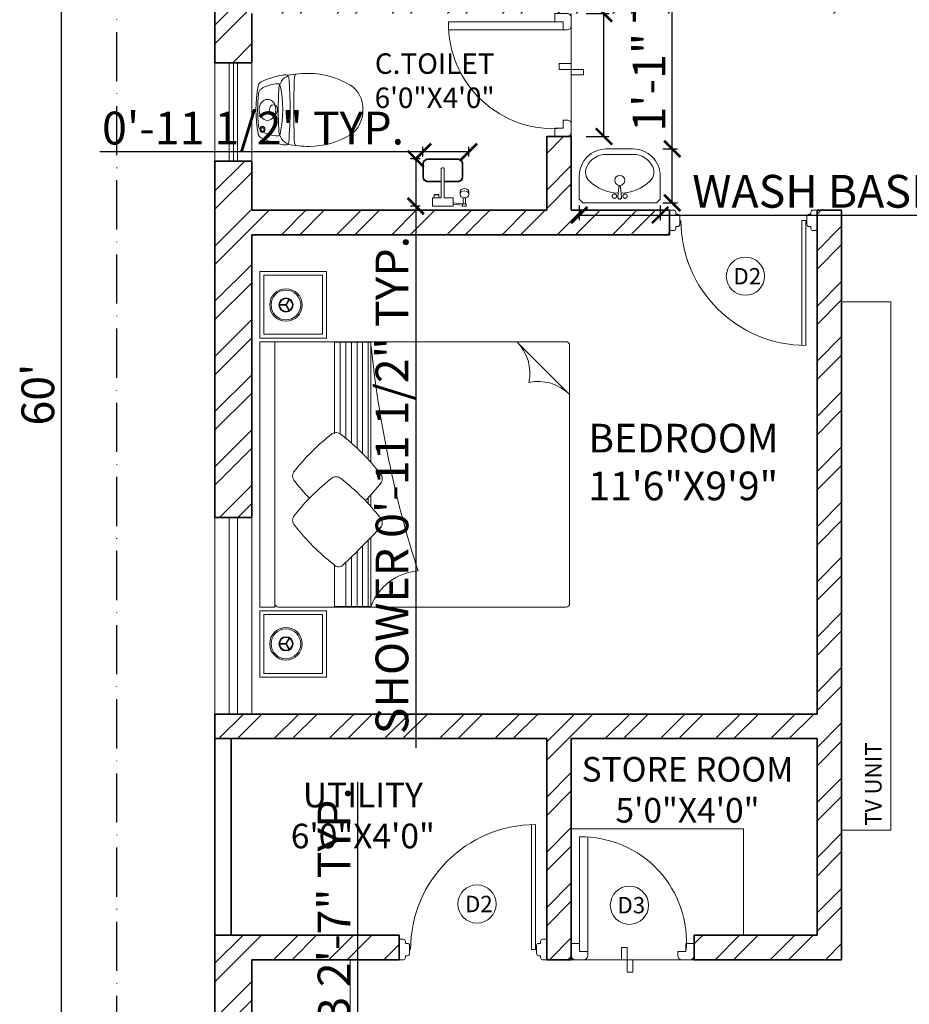
# Model space of a CAD drawing. Units: inches. Extents: x -15 to 1053, y -1 to 793.
# Tile 5 of 8: x 595 to 813, y 256 to 496. Entities that reach past the tile are written whole.
import ezdxf

# ---------------------------------------------------------------- set-up
doc = ezdxf.new("R2010")
doc.units = ezdxf.units.IN
doc.linetypes.add('ACAD_ISO10W100', pattern=[18, 12, -3, 0, -3])
for name, color, linetype, lineweight in [('00 FURNITURE', 15, 'Continuous', 15), ('A-ANNO-DIMS', 2, 'Continuous', 18), ('A-ANNO-TEXT', 7, 'Continuous', 18), ('A-AREA-IDEN', 7, 'Continuous', 18), ('A-DOOR', 4, 'Continuous', 18), ('A-FLOR-CASE', 5, 'Continuous', 18), ('A-FLOR-FIXT', 8, 'Continuous', 13), ('A-FURN', 8, 'Continuous', 13), ('A-GLAZ', 4, 'Continuous', 18), ('A-WALL', 7, 'Continuous', 35), ('A-WALL-PATT', 8, 'Continuous', 13), ('A_FUR 1', 5, 'Continuous', 5), ('C-PROP', 1, 'ACAD_ISO10W100', 25)]:
    doc.layers.add(name, color=color, linetype=linetype, lineweight=lineweight)
doc.styles.add('1-100DIM', font='txt', dxfattribs={"height": 0.3})
doc.styles.get("Standard").update_dxf_attribs({"font": 'arial.ttf'})
doc.dimstyles.new('ISO-25', dxfattribs={"dimtxt": 8, "dimasz": 4, "dimexe": 1.25, "dimexo": 0.625, "dimtad": 1, "dimdec": 0, "dimlunit": 4, "dimtxsty": 'Standard', "dimblk": 'ARCHTICK', "dimcen": 3, "dimadec": 0, "dimazin": 0, "dimtfac": 1, "dimtdec": 0, "dimtmove": 0, "dimatfit": 3, "dimldrblk": 'ARCHTICK', "dimfxl": 1, "dimarcsym": 0})

# ---------------------------------------------------------------- blocks, each defined once
blk = doc.blocks.new('_ArchTick')
at = {"color": 0, "linetype": 'ByBlock', "const_width": 0.15}
blk.add_lwpolyline([(-0.5, -0.5), (0.5, 0.5)], dxfattribs=at)
blk = doc.blocks.new('*D19')
at = {"layer": 'A-ANNO-DIMS', "color": 0, "lineweight": -2, "transparency": 16777216}
for p, q in [((618.45, 764.76), (604.32, 764.76)), ((605.57, 764.76), (605.57, 44.76)), ((618.45, 44.76), (604.32, 44.76))]:
    blk.add_line(p, q, dxfattribs=at)
at = {"layer": 'Defpoints', "color": 0, "transparency": 16777216}
for p in [(619.07, 764.76), (605.57, 44.76), (619.07, 44.76)]:
    blk.add_point(p, dxfattribs=at)
at = {"layer": 'A-ANNO-DIMS', "color": 0, "lineweight": -2, "transparency": 16777216, "xscale": 4, "yscale": 4, "zscale": 4}
for p, rotation in [((605.57, 764.76), 90), ((605.57, 44.76), 270)]:
    blk.add_blockref('_ArchTick', p, dxfattribs=dict(at, rotation=rotation))
at = {"layer": 'A-ANNO-DIMS', "color": 0, "transparency": 16777216, "insert": (600.86, 404.76), "char_height": 8, "attachment_point": 5, "rotation": 90}
blk.add_mtext("60'", dxfattribs=at)
blk = doc.blocks.new('ESTSET')
at = {"layer": 'A_FUR 1'}
for p, q in [((-10.44, 4.1), (-10.44, 32.1)), ((-8.44, 4.1), (-8.44, 32.1)), ((-36.44, 6.1), (-36.44, 3.1)), ((-34.44, 6.1), (-36.44, 6.1)), ((-34.44, 4.1), (-34.44, 6.1)), ((-34.44, 4.1), (-34.44, 6.1)), ((-8.44, 4.1), (-8.44, 6.1)), ((-8.44, 6.1), (-6.44, 6.1)), ((-8.44, 4.1), (-8.44, 6.1)), ((-6.44, 6.1), (-6.44, 3.1)), ((-32.44, 4.1), (-34.44, 4.1)), ((-32.44, 4.1), (-34.44, 4.1)), ((-32.44, 3.1), (-32.44, 4.1)), ((-10.44, 3.1), (-10.44, 4.1)), ((-10.44, 4.1), (-8.44, 4.1)), ((-10.44, 4.1), (-8.44, 4.1)), ((-6.44, 2.1), (-36.44, 2.1)), ((-35.44, 2.1), (-33.44, 2.1)), ((-7.44, 2.1), (-9.44, 2.1))]:
    blk.add_line(p, q, dxfattribs=at)
for points in [[(-21.44, 2.1), (-18.67, 2.1), (-18.67, 5.1), (-20.06, 5.1)], [(-20.06, 5.1), (-20.06, -0.91)], [(-21.44, 2.1), (-21.44, -0.91), (-20.06, -0.91)]]:
    blk.add_lwpolyline(points, dxfattribs=at)
for centre, radius, start, end in [((-8.91, 6.46), 25.64, 88.9606, 185.2816), ((-35.44, 3.1), 1, 180, 270), ((-33.44, 3.1), 1, 270, 0), ((-9.44, 3.1), 1, 180, 270), ((-7.44, 3.1), 1, 270, 0)]:
    blk.add_arc(centre, radius, start, end, dxfattribs=at)
blk = doc.blocks.new('RGWTG')
at = {"layer": '00 FURNITURE'}
for p, q in [((578.23, 3473.51), (577.36, 3475.01)), ((578.23, 3473.58), (577.36, 3472.08)), ((578.36, 3473.58), (577.49, 3475.09)), ((578.29, 3473.62), (580.03, 3473.62)), ((578.36, 3473.51), (577.49, 3472)), ((578.29, 3473.47), (580.03, 3473.47)), ((521.93, 3464.58), (509.03, 3451.68)), ((509.93, 3464.58), (566.4, 3464.58)), ((557.53, 3463.84), (557.53, 3464.49)), ((557.53, 3464.49), (566.4, 3464.49)), ((558.2, 3464.49), (558.2, 3435.82)), ((559.57, 3464.49), (559.57, 3437.25)), ((560.94, 3464.49), (560.94, 3438.58)), ((562.3, 3464.49), (562.3, 3439.83)), ((563.67, 3464.49), (563.67, 3440.99)), ((565.04, 3464.49), (565.04, 3442.08)), ((566.4, 3464.58), (580.98, 3464.58)), ((566.4, 3464.49), (566.4, 3442.08)), ((566.4, 3464.49), (566.4, 3463.84)), ((580.98, 3464.58), (580.98, 3416.72)), ((509.03, 3422.63), (509.03, 3463.68)), ((558.2, 3426.48), (558.2, 3425.04)), ((509.03, 3400.68), (509.03, 3422.63)), ((558.2, 3416.13), (558.2, 3399.95)), ((580.98, 3416.72), (580.98, 3400.68)), ((559.57, 3414.75), (559.57, 3399.95)), ((560.94, 3413.39), (560.94, 3399.95)), ((562.3, 3412.04), (562.3, 3399.95)), ((563.67, 3410.72), (563.67, 3399.95)), ((580.08, 3399.78), (509.93, 3399.78)), ((557.53, 3399.95), (557.53, 3400.6)), ((566.4, 3399.95), (557.53, 3399.95)), ((566.4, 3400.6), (566.4, 3399.95)), ((578.23, 3390.78), (577.36, 3392.29)), ((578.36, 3390.86), (577.49, 3392.36)), ((578.23, 3390.86), (577.36, 3389.36)), ((578.36, 3390.78), (577.49, 3389.28)), ((578.29, 3390.9), (580.03, 3390.9)), ((578.29, 3390.74), (580.03, 3390.74))]:
    blk.add_line(p, q, dxfattribs=at)
for points in [[(568.43, 3465.48), (584.63, 3465.48), (584.63, 3481.68), (568.43, 3481.68)], [(569.33, 3466.38), (583.73, 3466.38), (583.73, 3480.78), (569.33, 3480.78)], [(580.98, 3399.78), (584.63, 3399.78), (584.63, 3464.58), (580.98, 3464.58)], [(568.43, 3398.88), (584.63, 3398.88), (584.63, 3382.68), (568.43, 3382.68)], [(569.33, 3397.98), (583.73, 3397.98), (583.73, 3383.58), (569.33, 3383.58)]]:
    blk.add_lwpolyline(points, close=True, dxfattribs=at)
for points in [[(566.52, 3464.49), (557.53, 3464.49), (557.53, 3435.08)], [(557.53, 3427.21), (557.53, 3424.3)], [(557.53, 3416.82), (557.53, 3399.95), (566.4, 3399.95), (566.4, 3409.94)]]:
    blk.add_lwpolyline(points, dxfattribs=at)
for centre, radius in [((578.29, 3473.54), 3.97), ((578.29, 3473.54), 3.63), ((578.29, 3473.54), 1.74), ((578.29, 3473.54), 1.56), ((578.29, 3390.82), 3.97), ((578.29, 3390.82), 3.63), ((578.29, 3390.82), 1.74), ((578.29, 3390.82), 1.56)]:
    blk.add_circle(centre, radius, dxfattribs=at)
for centre, radius, start, end in [((509.93, 3463.68), 0.9, 90, 180), ((529.65, 3456.88), 10.9, 135.0361, 191.9278), ((290.56, 3490.52), 268.3, 342.2214, 354.2925), ((516.73, 3443.97), 10.9, 78.0722, 134.9639), ((566.05, 3440.57), 1.82, 45, 135), ((598.15, 3399.01), 54.32, 127.931, 142.069), ((533.58, 3399.31), 54.32, 37.931, 52.069), ((574.84, 3431.77), 1.82, 315, 45), ((556.59, 3431.11), 1.82, 135, 225), ((598.15, 3388.23), 54.32, 127.931, 142.069), ((566.05, 3429.78), 1.82, 45, 135), ((533.58, 3388.53), 54.32, 37.931, 52.069), ((533.28, 3463.88), 54.32, 316.32, 322.069), ((597.87, 3463.6), 54.32, 217.931, 224.141), ((556.59, 3420.33), 1.82, 135, 225), ((574.84, 3420.99), 1.82, 315, 45), ((765.33, 3619.75), 290.45, 223.6069, 226.2326), ((533.28, 3453.1), 54.32, 307.931, 322.069), ((565.44, 3411.05), 1.47, 225.9674, 326.8337), ((545.02, 3395.29), 13.35, 20.4224, 85.5825), ((509.93, 3400.68), 0.9, 180, 270), ((580.08, 3400.68), 0.9, 270, 0)]:
    blk.add_arc(centre, radius, start, end, dxfattribs=at)
blk = doc.blocks.new('s_14')
at = {"extrusion": (0, 0, -1)}
for centre, major_axis, start_param, end_param in [((-0.2, -522.3), (652.4, -0.3), 4.476887, 4.947891), ((-0.2, -522.3), (652.4, -0.3), 4.476887, 4.947891), ((681.3, -278.7), (913.7, -0.4), 3.289642, 3.481728), ((681.3, -278.7), (913.7, -0.4), 3.289642, 3.481728), ((-143.1, -44.8), (39.1, 0), 3.481728, 4.476887), ((-143.1, -44.8), (39.1, 0), 3.481728, 4.476887), ((118.1, -139.4), (284.9, -0.1), 3.130806, 3.616946), ((-125.1, -42.1), (19.2, 0), 3.141593, 9.424778), ((-125.1, -42.1), (12.2, 0), 3.141593, 9.424778), ((-97.4, -50.5), (42.5, 0), 3.616946, 4.577347), ((-0.3, -624.1), (765.5, -0.4), 4.577347, 4.847431), ((0, -73.8), (67.1, 0), 3.141593, 9.424778), ((97.3, -50.6), (42.5, 0), -1.435755, -0.475353), ((-118.3, -139.3), (284.9, -0.1), -0.475353, 0.010787), ((143.1, -44.9), (39.1, 0), -1.335294, -0.340135), ((143.1, -44.9), (39.1, 0), -1.335294, -0.340135), ((-681.5, -278.1), (913.7, -0.4), -0.340135, -0.148049), ((-681.5, -278.1), (913.7, -0.4), -0.340135, -0.148049), ((-0.1, -112.6), (32.9, 0), 3.141593, 9.424778), ((-87.1, -186.6), (136.8, -0.1), 3.032389, 3.289642), ((-87.1, -186.6), (136.8, -0.1), 3.032389, 3.289642), ((-120.9, -224.6), (98.7, 0), 3.365215, 4.657014), ((-148.9, -141.6), (17.9, 0), 1.839297, 3.130806), ((0.1, 291.4), (579, -0.3), 1.302296, 1.839297), ((-0.9, -1969.6), (2281.8, -1.1), 4.657014, 4.767764), ((120.7, -224.8), (98.7, 0), -1.515421, -0.223622), ((148.8, -141.7), (17.9, 0), 0.010787, 1.302296), ((86.9, -186.7), (136.8, -0.1), -0.148049, 0.109204), ((86.9, -186.7), (136.8, -0.1), -0.148049, 0.109204), ((999.2, -341.8), (1233.1, -0.6), 3.141593, 3.282422), ((999.2, -341.8), (1233.1, -0.6), 3.141593, 3.282422), ((-210, -262.6), (19.7, 0), 3.222651, 4.658459), ((-207.2, -197.1), (16, 0), 1.680926, 3.032389), ((-207.2, -197.1), (16, 0), 1.680926, 3.032389), ((-1.6, -3375.8), (3914.3, -1.8), 4.658459, 4.766319), ((0.6, 1302.1), (1900.3, -0.9), 1.460666, 1.680926), ((0.6, 1302.1), (1900.3, -0.9), 1.460666, 1.680926), ((207, -197.3), (16, 0), 0.109204, 1.460666), ((207, -197.3), (16, 0), 0.109204, 1.460666), ((209.8, -262.8), (19.7, 0), -1.516867, -0.081058), ((-999.6, -340.9), (1233.1, -0.6), -0.140829, 0), ((-999.6, -340.9), (1233.1, -0.6), -0.140829, 0), ((526.7, -341.6), (760.5, -0.4), 2.693443, 3.141593), ((526.7, -341.6), (760.5, -0.4), 2.693443, 3.141593), ((-527, -341.1), (760.5, -0.4), 0, 0.44815), ((-527, -341.1), (760.5, -0.4), 0, 0.44815), ((-0.3, -544.1), (175.9, -0.1), 0.44815, 2.693443), ((-0.3, -544.1), (175.9, -0.1), 0.44815, 2.693443)]:
    blk.add_ellipse(centre, major_axis=major_axis, ratio=0.800511, start_param=start_param, end_param=end_param, dxfattribs=at)
blk = doc.blocks.new('s_46')
at = {"ltscale": 600}
h = blk.add_hatch(color=256, dxfattribs=at)
edge = h.paths.add_edge_path()
edge.add_line((13.5, 62), (14.2, 54.1))
edge.add_ellipse((4.2, 52.3), major_axis=(-10.1, 0), ratio=1, start_angle=540, end_angle=550.1755, ccw=False)
edge.add_arc((4.2, 52.3), 10.1, 270, 360, ccw=False)
edge.add_line((4.2, 42.2), (4.2, 41.3))
edge.add_line((4.2, 41.3), (11.9, 41.3))
edge.add_arc((4.2, 52.3), 13.4, 664.6981, 766.4848)
h.paths.add_polyline_path([(4.2, 41.3), (-3.4, 41.3, 0.152567), (4.2, 38.9)])
h.paths.add_polyline_path([(11.9, 41.3), (4.2, 41.3), (4.2, 38.9, 0.152567)])
h.paths.add_polyline_path([(-5.7, 54.1), (-5, 62, 0.475833), (-3.4, 41.3), (4.2, 41.3), (4.2, 42.2, -0.46724)])
for p, q in [((-5.9, 52.3), (-0.7, 110.5)), ((-5.9, 52.3), (-0.7, 110.5)), ((9.1, 110.5), (14.2, 54.1)), ((14.3, 52.3), (9.1, 110.5)), ((14.2, 54.1), (14.3, 52.3))]:
    blk.add_line(p, q, dxfattribs=at)
blk.add_lwpolyline([(-220.8, 171.3, -0.414214), (-70.8, 321.3), (79.2, 321.3, -0.414214), (229.2, 171.3), (229.2, 41.3), (209.2, 21.3), (-200.8, 21.3), (-220.8, 41.3)], format="xyb", close=True, dxfattribs=at)
blk.add_lwpolyline([(12.3, 75.4, 0.181638), (172.2, 141.5, 0.326351), (187.7, 222.7, 0.289814), (79.2, 291.3), (-70.8, 291.3, 0.289814), (-179.2, 222.7, 0.326351), (-163.8, 141.5, 0.181638), (-3.8, 75.4)], format="xyb", dxfattribs=at)
for points in [[(-16.8, 67.4), (-17, 67.5), (-17.2, 67.6), (-17.4, 67.6), (-17.6, 67.7), (-17.8, 67.8), (-18, 67.9), (-18.1, 68.1), (-18.2, 68.2), (-18.3, 68.4), (-18.4, 68.6), (-18.5, 68.8), (-18.7, 68.9), (-18.8, 69.1), (-18.9, 69.2), (-19.1, 69.3), (-19.3, 69.3), (-19.5, 69.3), (-19.7, 69.4), (-19.9, 69.4), (-20.1, 69.4), (-20.3, 69.4), (-20.5, 69.5), (-20.7, 69.6), (-20.8, 69.7), (-21, 69.9), (-21.1, 70), (-21.3, 70.2), (-21.4, 70.3), (-21.5, 70.4), (-21.7, 70.5), (-21.9, 70.5), (-22.1, 70.5), (-22.3, 70.5), (-22.5, 70.5), (-22.7, 70.4), (-22.9, 70.4), (-23.1, 70.4), (-23.3, 70.4), (-23.5, 70.5), (-23.7, 70.6), (-23.9, 70.7), (-24, 70.8), (-24.2, 70.9), (-24.4, 71), (-24.6, 71.1), (-24.7, 71.1), (-24.9, 71.1), (-25.1, 71), (-25.3, 71), (-25.5, 70.9), (-25.7, 70.8), (-25.9, 70.7), (-26.1, 70.6), (-26.3, 70.6), (-26.5, 70.6), (-26.7, 70.6), (-26.9, 70.7), (-27.1, 70.8), (-27.3, 70.8), (-27.5, 70.9), (-27.7, 70.9), (-27.8, 70.9), (-28, 70.8), (-28.2, 70.8), (-28.3, 70.6), (-28.5, 70.5), (-28.7, 70.4), (-28.9, 70.3), (-29.1, 70.2), (-29.3, 70.1), (-29.6, 70.1), (-29.9, 70.1), (-30.2, 70.1), (-30.5, 70), (-30.8, 69.8), (-31.1, 69.5), (-31.4, 69), (-31.6, 68.4), (-32.3, 68.5), (-32.8, 68.4), (-33.2, 68.3), (-33.5, 68.1), (-33.7, 67.8), (-33.9, 67.6), (-34, 67.3), (-34.1, 67.1), (-34.3, 66.9), (-34.5, 66.7), (-34.7, 66.6), (-34.9, 66.5), (-35.1, 66.4), (-35.2, 66.3), (-35.4, 66.2), (-35.5, 66), (-35.6, 65.9), (-35.6, 65.7), (-35.7, 65.5), (-35.7, 65.3), (-35.7, 65.1), (-35.8, 64.9), (-35.8, 64.7), (-35.9, 64.5), (-36, 64.3), (-36.2, 64.2), (-36.3, 64), (-36.5, 63.9), (-36.6, 63.8), (-36.8, 63.6), (-36.9, 63.5), (-37, 63.3), (-37, 63.1), (-37, 63), (-37, 62.8), (-37, 62.6), (-37, 62.3), (-37, 62.1), (-37, 61.9), (-37, 61.7), (-37.1, 61.5), (-37.2, 61.4), (-37.3, 61.2), (-37.4, 61), (-37.5, 60.8), (-37.6, 60.7), (-37.7, 60.5), (-37.8, 60.3), (-37.8, 60.1), (-37.7, 60), (-37.7, 59.8), (-37.6, 59.6), (-37.5, 59.4), (-37.4, 59.2), (-37.4, 59), (-37.4, 58.8), (-37.4, 58.6), (-37.4, 58.4), (-37.5, 58.2), (-37.6, 58), (-37.7, 57.8), (-37.7, 57.6), (-37.8, 57.4), (-37.8, 57.2), (-37.7, 57.1), (-37.6, 56.9), (-37.5, 56.7), (-37.4, 56.6), (-37.3, 56.4), (-37.2, 56.2), (-37.1, 56), (-37, 55.8), (-37, 55.6), (-37, 55.4), (-37, 55.2), (-37, 55), (-37, 54.8), (-37, 54.6), (-37, 54.4), (-37, 54.2), (-36.9, 54.1), (-36.8, 53.9), (-36.6, 53.8), (-36.5, 53.7), (-36.3, 53.5), (-36.2, 53.4), (-36, 53.2), (-35.9, 53.1), (-35.8, 52.9), (-35.8, 52.7), (-35.7, 52.5), (-35.7, 52.3), (-35.7, 52.1), (-35.6, 51.9), (-35.6, 51.7), (-35.5, 51.5), (-35.4, 51.4), (-35.2, 51.3), (-35.1, 51.2), (-34.9, 51.1), (-34.7, 51), (-34.5, 50.9), (-34.3, 50.8), (-34.2, 50.7), (-34, 50.5), (-33.9, 50.3), (-33.8, 50.1), (-33.8, 49.9), (-33.7, 49.8), (-33.6, 49.6), (-33.5, 49.4), (-33.4, 49.3), (-33.2, 49.2), (-33.1, 49.1), (-32.9, 49.1), (-32.7, 49), (-32.5, 49), (-32.2, 48.9), (-32.1, 48.9), (-31.9, 48.8), (-31.7, 48.7), (-31.6, 48.5), (-31.4, 48.3), (-31.3, 48.2), (-31.2, 48), (-31.1, 47.9), (-30.9, 47.7), (-30.8, 47.6), (-30.6, 47.6), (-30.4, 47.5), (-30.2, 47.5), (-30, 47.6), (-29.8, 47.6), (-29.6, 47.6), (-29.4, 47.6), (-29.2, 47.5), (-29, 47.4), (-28.8, 47.3), (-28.7, 47.2), (-28.5, 47.1), (-28.3, 46.9), (-28.2, 46.8), (-28, 46.7), (-27.8, 46.7), (-27.7, 46.7), (-27.5, 46.7), (-27.3, 46.7), (-27.1, 46.8), (-26.9, 46.9), (-26.7, 46.9), (-26.5, 47), (-26.3, 47), (-26.1, 46.9), (-25.9, 46.9), (-25.7, 46.8), (-25.5, 46.7), (-25.3, 46.6), (-25.1, 46.5), (-24.9, 46.5), (-24.7, 46.5), (-24.6, 46.5), (-24.4, 46.6), (-24.2, 46.7), (-24, 46.8), (-23.9, 46.9), (-23.7, 47), (-23.5, 47.1), (-23.3, 47.1), (-23.1, 47.2), (-22.9, 47.2), (-22.7, 47.1), (-22.5, 47.1), (-22.3, 47), (-22.1, 47), (-21.9, 47), (-21.7, 47.1), (-21.5, 47.1), (-21.4, 47.2), (-21.3, 47.4), (-21.1, 47.5), (-21, 47.7), (-20.8, 47.8), (-20.7, 48), (-20.5, 48.1), (-20.3, 48.1), (-20.1, 48.2), (-19.9, 48.2), (-19.7, 48.2), (-19.5, 48.2), (-19.3, 48.2), (-19.1, 48.3), (-18.9, 48.4), (-18.8, 48.5), (-18.7, 48.6), (-18.5, 48.8), (-18.4, 49), (-18.3, 49.2), (-18.2, 49.3), (-18.1, 49.5), (-18, 49.7), (-17.8, 49.8), (-17.6, 49.9), (-17.4, 49.9), (-17.2, 50), (-17, 50.1), (-16.8, 50.1), (-16.7, 50.2), (-16.5, 50.3), (-16.4, 50.5), (-16.3, 50.7), (-16.3, 50.8), (-16.2, 51), (-16.2, 51.3), (-16.1, 51.5), (-16, 51.6), (-15.9, 51.8), (-15.8, 52), (-15.6, 52.1), (-15.5, 52.2), (-15.3, 52.3), (-15.1, 52.4), (-15, 52.6), (-14.8, 52.7), (-14.7, 52.8), (-14.7, 53), (-14.6, 53.2), (-14.6, 53.4), (-14.6, 53.6), (-14.6, 53.8), (-14.6, 54), (-14.6, 54.2), (-14.5, 54.4), (-14.4, 54.6), (-14.3, 54.8), (-14.2, 54.9), (-14, 55.1), (-13.9, 55.2), (-13.7, 55.4), (-13.6, 55.5), (-13.6, 55.7), (-13.6, 55.9), (-13.6, 56.1), (-13.6, 56.3), (-13.7, 56.5), (-13.7, 56.7), (-13.8, 56.9), (-13.8, 57.1), (-13.8, 57.3), (-13.7, 57.5), (-13.7, 57.7), (-13.6, 57.9), (-13.5, 58.1), (-13.4, 58.2), (-13.3, 58.4), (-13.2, 58.6), (-13.2, 58.8), (-13.2, 59), (-13.3, 59.1), (-13.4, 59.3), (-13.5, 59.5), (-13.6, 59.7), (-13.7, 59.9), (-13.7, 60.1), (-13.8, 60.3), (-13.8, 60.5), (-13.8, 60.7), (-13.7, 60.9), (-13.7, 61.1), (-13.6, 61.3), (-13.6, 61.5), (-13.6, 61.7), (-13.6, 61.9), (-13.6, 62), (-13.7, 62.2), (-13.9, 62.3), (-14, 62.5), (-14.2, 62.6), (-14.3, 62.8), (-14.4, 63), (-14.5, 63.1), (-14.6, 63.3), (-14.6, 63.5), (-14.6, 63.8), (-14.6, 64), (-14.6, 64.2), (-14.6, 64.4), (-14.7, 64.6), (-14.7, 64.7), (-14.8, 64.9), (-15, 65), (-15.1, 65.1), (-15.3, 65.2), (-15.5, 65.3), (-15.6, 65.5), (-15.8, 65.6), (-15.9, 65.7), (-16, 65.9), (-16.1, 66.1), (-16.2, 66.3), (-16.2, 66.5), (-16.3, 66.7), (-16.3, 66.9), (-16.4, 67.1), (-16.5, 67.2), (-16.7, 67.3)], [(22.1, 61.1), (22, 61.3), (22, 61.5), (22, 61.7), (22, 61.9), (22.1, 62), (22.2, 62.2), (22.3, 62.3), (22.4, 62.5), (22.6, 62.6), (22.7, 62.8), (22.8, 63), (22.9, 63.1), (23, 63.3), (23, 63.5), (23, 63.8), (23, 64), (23, 64.2), (23, 64.4), (23.1, 64.6), (23.1, 64.7), (23.2, 64.9), (23.4, 65), (23.5, 65.1), (23.7, 65.2), (23.9, 65.3), (24.1, 65.5), (24.2, 65.6), (24.4, 65.7), (24.5, 65.9), (24.5, 66.1), (24.6, 66.3), (24.7, 66.5), (24.7, 66.7), (24.8, 66.9), (24.9, 67.1), (25, 67.2), (25.1, 67.3), (25.3, 67.4), (25.4, 67.5), (25.6, 67.6), (25.8, 67.6), (26, 67.7), (26.2, 67.8), (26.4, 67.9), (26.5, 68.1), (26.7, 68.2), (26.8, 68.4), (26.9, 68.6), (27, 68.8), (27.1, 68.9), (27.2, 69.1), (27.3, 69.2), (27.5, 69.3), (27.7, 69.3), (27.9, 69.3), (28.1, 69.4), (28.3, 69.4), (28.5, 69.4), (28.7, 69.4), (28.9, 69.5), (29.1, 69.6), (29.2, 69.7), (29.4, 69.9), (29.5, 70), (29.7, 70.2), (29.8, 70.3), (30, 70.4), (30.1, 70.5), (30.3, 70.5), (30.5, 70.5), (30.7, 70.5), (30.9, 70.5), (31.1, 70.4), (31.3, 70.4), (31.5, 70.4), (31.7, 70.4), (31.9, 70.5), (32.1, 70.6), (32.3, 70.7), (32.5, 70.8), (32.6, 70.9), (32.8, 71), (33, 71.1), (33.2, 71.1), (33.4, 71.1), (33.5, 71), (33.7, 71), (33.9, 70.9), (34.1, 70.8), (34.3, 70.7), (34.5, 70.6), (34.7, 70.6), (34.9, 70.6), (35.1, 70.6), (35.3, 70.7), (35.5, 70.8), (35.7, 70.8), (35.9, 70.9), (36.1, 70.9), (36.3, 70.9), (36.4, 70.8), (36.6, 70.8), (36.8, 70.6), (36.9, 70.5), (37.1, 70.4), (37.3, 70.3), (37.5, 70.2), (37.8, 70.1), (38, 70.1), (38.3, 70.1), (38.6, 70.1), (38.9, 70), (39.2, 69.8), (39.5, 69.5), (39.8, 69), (40.1, 68.4), (40.7, 68.5), (41.3, 68.4), (41.7, 68.3), (42, 68.1), (42.2, 67.8), (42.3, 67.6), (42.4, 67.3), (42.6, 67.1), (42.7, 66.9), (42.9, 66.7), (43.1, 66.6), (43.3, 66.5), (43.5, 66.4), (43.6, 66.3), (43.8, 66.2), (43.9, 66), (44, 65.9), (44.1, 65.7), (44.1, 65.5), (44.1, 65.3), (44.2, 65.1), (44.2, 64.9), (44.2, 64.7), (44.3, 64.5), (44.4, 64.3), (44.6, 64.2), (44.7, 64), (44.9, 63.9), (45.1, 63.8), (45.2, 63.6), (45.3, 63.5), (45.4, 63.3), (45.5, 63.1), (45.5, 63), (45.5, 62.8), (45.4, 62.6), (45.4, 62.3), (45.4, 62.1), (45.4, 61.9), (45.4, 61.7), (45.5, 61.5), (45.6, 61.4), (45.7, 61.2), (45.8, 61), (46, 60.8), (46.1, 60.7), (46.1, 60.5), (46.2, 60.3), (46.2, 60.1), (46.1, 60), (46.1, 59.8), (46, 59.6), (45.9, 59.4), (45.9, 59.2), (45.8, 59), (45.8, 58.8), (45.8, 58.6), (45.9, 58.4), (45.9, 58.2), (46, 58), (46.1, 57.8), (46.1, 57.6), (46.2, 57.4), (46.2, 57.2), (46.1, 57.1), (46.1, 56.9), (46, 56.7), (45.8, 56.6), (45.7, 56.4), (45.6, 56.2), (45.5, 56), (45.4, 55.8), (45.4, 55.6), (45.4, 55.4), (45.4, 55.2), (45.4, 55), (45.5, 54.8), (45.5, 54.6), (45.5, 54.4), (45.4, 54.2), (45.3, 54.1), (45.2, 53.9), (45.1, 53.8), (44.9, 53.7), (44.7, 53.5), (44.6, 53.4), (44.4, 53.2), (44.3, 53.1), (44.2, 52.9), (44.2, 52.7), (44.2, 52.5), (44.1, 52.3), (44.1, 52.1), (44.1, 51.9), (44, 51.7), (43.9, 51.5), (43.8, 51.4), (43.6, 51.3), (43.5, 51.2), (43.3, 51.1), (43.1, 51), (42.9, 50.9), (42.7, 50.8), (42.6, 50.7), (42.5, 50.5), (42.4, 50.3), (42.3, 50.1), (42.2, 49.9), (42.1, 49.8), (42, 49.6), (41.9, 49.4), (41.8, 49.3), (41.7, 49.2), (41.5, 49.1), (41.3, 49.1), (41.1, 49), (40.9, 49), (40.7, 48.9), (40.5, 48.9), (40.3, 48.8), (40.1, 48.7), (40, 48.5), (39.9, 48.3), (39.7, 48.2), (39.6, 48), (39.5, 47.9), (39.4, 47.7), (39.2, 47.6), (39, 47.6), (38.8, 47.5), (38.6, 47.5), (38.4, 47.6), (38.2, 47.6), (38, 47.6), (37.8, 47.6), (37.6, 47.5), (37.4, 47.4), (37.2, 47.3), (37.1, 47.2), (36.9, 47.1), (36.8, 46.9), (36.6, 46.8), (36.4, 46.7), (36.3, 46.7), (36.1, 46.7), (35.9, 46.7), (35.7, 46.7), (35.5, 46.8), (35.3, 46.9), (35.1, 46.9), (34.9, 47), (34.7, 47), (34.5, 46.9), (34.3, 46.9), (34.1, 46.8), (33.9, 46.7), (33.7, 46.6), (33.5, 46.5), (33.4, 46.5), (33.2, 46.5), (33, 46.5), (32.8, 46.6), (32.6, 46.7), (32.5, 46.8), (32.3, 46.9), (32.1, 47), (31.9, 47.1), (31.7, 47.1), (31.5, 47.2), (31.3, 47.2), (31.1, 47.1), (30.9, 47.1), (30.7, 47), (30.5, 47), (30.3, 47), (30.1, 47.1), (30, 47.1), (29.8, 47.2), (29.7, 47.4), (29.5, 47.5), (29.4, 47.7), (29.2, 47.8), (29.1, 48), (28.9, 48.1), (28.7, 48.1), (28.5, 48.2), (28.3, 48.2), (28.1, 48.2), (27.9, 48.2), (27.7, 48.2), (27.5, 48.3), (27.3, 48.4), (27.2, 48.5), (27.1, 48.6), (27, 48.8), (26.9, 49), (26.8, 49.2), (26.7, 49.3), (26.5, 49.5), (26.4, 49.7), (26.2, 49.8), (26, 49.9), (25.8, 49.9), (25.6, 50), (25.4, 50.1), (25.3, 50.1), (25.1, 50.2), (25, 50.3), (24.9, 50.5), (24.8, 50.7), (24.7, 50.8), (24.7, 51), (24.6, 51.3), (24.5, 51.5), (24.5, 51.6), (24.4, 51.8), (24.2, 52), (24.1, 52.1), (23.9, 52.2), (23.7, 52.3), (23.5, 52.4), (23.4, 52.6), (23.2, 52.7), (23.1, 52.8), (23.1, 53), (23, 53.2), (23, 53.4), (23, 53.6), (23, 53.8), (23, 54), (23, 54.2), (22.9, 54.4), (22.8, 54.6), (22.7, 54.8), (22.6, 54.9), (22.4, 55.1), (22.3, 55.2), (22.2, 55.4), (22.1, 55.5), (22, 55.7), (22, 55.9), (22, 56.1), (22, 56.3), (22.1, 56.5), (22.1, 56.7), (22.2, 56.9), (22.2, 57.1), (22.2, 57.3), (22.2, 57.5), (22.1, 57.7), (22, 57.9), (21.9, 58.1), (21.8, 58.2), (21.7, 58.4), (21.6, 58.6), (21.6, 58.8), (21.6, 59), (21.7, 59.1), (21.8, 59.3), (21.9, 59.5), (22, 59.7), (22.1, 59.9), (22.2, 60.1), (22.2, 60.3), (22.2, 60.5), (22.2, 60.7), (22.1, 60.9)]]:
    blk.add_lwpolyline(points, close=True, dxfattribs=at)
blk.add_circle((4.2, 146.3), 28, dxfattribs=at)
for centre, radius, start, end in [((4.2, 108.2), 5.42, 24.6783, 155.3217), ((4.2, 52.3), 10.1, 169.8245, 0)]:
    blk.add_arc(centre, radius, start, end, dxfattribs=at)
for centre, major_axis, ratio, start_param, end_param in [((4.2, 110.5), (-4.93, 0), 0.641024, 3.141593, 6.283185), ((4.2, 52.3), (-10.1, 0), 1, 6.10559, 9.602373)]:
    blk.add_ellipse(centre, major_axis=major_axis, ratio=ratio, start_param=start_param, end_param=end_param, dxfattribs=at)
blk = doc.blocks.new('A$C7A0926BE')
for p, q in [((-6.55, 0), (-5.57, 0)), ((-6.55, -0.65), (-6.55, 0)), ((-5.57, 0), (-5.57, -0.65)), ((-2.89, 0), (-2.89, -2.29)), ((2.89, 0), (-2.89, 0)), ((2.89, -2.29), (2.89, 0)), ((-5.57, -0.65), (-6.55, -0.65)), ((-6.34, -0.65), (-5.74, -0.65)), ((-6.34, -2.33), (-6.34, -0.65)), ((-5.74, -2.33), (-6.34, -2.33)), ((-5.74, -0.65), (-5.74, -2.33)), ((-5.57, -0.28), (-2.89, -0.56)), ((-5.57, -0.65), (-2.89, -0.94)), ((-2.89, -2.29), (-0.45, -2.29)), ((0.39, -2.29), (2.89, -2.29)), ((1.04, -2.29), (1.04, -3.12)), ((2.37, -2.29), (1.04, -2.29)), ((2.37, -3.12), (2.37, -2.29)), ((-7.32, -3.29), (-7.32, -3.94)), ((-4.84, -3.94), (-4.85, -3.29)), ((1.04, -3.12), (2.37, -3.12)), ((1.13, -3.12), (1.13, -3.23)), ((2.3, -3.12), (1.13, -3.12)), ((1.13, -3.23), (2.3, -3.23)), ((2.3, -3.23), (2.3, -3.12))]:
    blk.add_line(p, q)
at = {"ltscale": 100}
for p, q in [((-0.45, -10.48), (-0.45, -2.29)), ((0.39, -10.48), (0.39, -2.29)), ((0.18, -10.69), (-0.24, -10.69))]:
    blk.add_line(p, q, dxfattribs=at)
for points in [[(-0.45, -6.79), (-4.23, -6.79, 0.414214), (-5.63, -8.19), (-5.63, -11.8, 0.414214), (-4.23, -13.2), (4.17, -13.2, 0.414214), (5.57, -11.8), (5.57, -8.19, 0.414214), (4.17, -6.79), (0.39, -6.79)], [(-0.45, -7), (-4.23, -7, 0.414214), (-5.42, -8.19), (-5.42, -11.8, 0.414214), (-4.23, -12.99), (4.17, -12.99, 0.414214), (5.36, -11.8), (5.36, -8.19, 0.414214), (4.17, -7), (0.39, -7)]]:
    blk.add_lwpolyline(points, format="xyb", dxfattribs=at)
for centre, start, end in [((-0.24, -10.48), 180, 270), ((0.18, -10.48), 270, 0)]:
    blk.add_arc(centre, 0.21, start, end, dxfattribs=at)
at = {"extrusion": (0, 0, -1)}
blk.add_ellipse((-6.08, -3.29), major_axis=(-1.24, 0), ratio=0.790849, dxfattribs=at)
blk.add_ellipse((-6.08, -3.94), major_axis=(-1.24, 0), ratio=0.790849, start_param=3.141593, end_param=6.283185, dxfattribs=at)
blk = doc.blocks.new('DDD')
at = {"layer": '00 FURNITURE'}
for p, q in [((-12579.77, -15859.53), (-12579.77, -15829.05)), ((-12578.77, -15859.53), (-12578.77, -15829.03)), ((-12612.02, -15857.03), (-12612.02, -15862.03)), ((-12611.02, -15857.03), (-12612.02, -15857.03)), ((-12610.52, -15858.03), (-12610.52, -15857.53)), ((-12577.52, -15858.03), (-12577.52, -15857.53)), ((-12577.02, -15857.03), (-12576.02, -15857.03)), ((-12576.02, -15857.03), (-12576.02, -15862.03)), ((-12578.77, -15859.53), (-12579.77, -15859.53)), ((-12612.02, -15862.03), (-12611.02, -15862.03)), ((-12610.52, -15861.53), (-12610.52, -15861.03)), ((-12577.52, -15861.53), (-12577.52, -15861.03)), ((-12576.02, -15862.03), (-12577.02, -15862.03))]:
    blk.add_line(p, q, dxfattribs=at)
for points in [[(-12610.52, -15861.03), (-12610.02, -15861.03, 0.414214), (-12609.52, -15860.53), (-12609.52, -15858.53, 0.414214), (-12610.02, -15858.03), (-12610.52, -15858.03)], [(-12577.52, -15861.03), (-12578.02, -15861.03, -0.414214), (-12578.52, -15860.53), (-12578.52, -15858.53, -0.414214), (-12578.02, -15858.03), (-12577.52, -15858.03)]]:
    blk.add_lwpolyline(points, format="xyb", dxfattribs=at)
for centre, radius, start, end in [((-12578.77, -15859.53), 30.5, 90, 180), ((-12611.02, -15857.53), 0.5, 0, 90), ((-12577.02, -15857.53), 0.5, 90, 180), ((-12611.02, -15861.53), 0.5, 270, 0), ((-12577.02, -15861.53), 0.5, 180, 270)]:
    blk.add_arc(centre, radius, start, end, dxfattribs=at)
blk = doc.blocks.new('*D36')
at = {"layer": 'A-ANNO-DIMS', "color": 0, "lineweight": -2, "transparency": 16777216}
for p, q in [((699.94, 502.73), (609.69, 502.73)), ((699.94, 498.39), (699.94, 503.98)), ((733.08, 502.73), (699.94, 502.73)), ((733.08, 498.39), (733.08, 503.98))]:
    blk.add_line(p, q, dxfattribs=at)
at = {"layer": 'Defpoints', "color": 0, "transparency": 16777216}
for p in [(699.94, 502.73), (699.94, 497.76), (733.08, 497.76)]:
    blk.add_point(p, dxfattribs=at)
at = {"layer": 'A-ANNO-DIMS', "color": 0, "lineweight": -2, "transparency": 16777216, "xscale": 4, "yscale": 4, "zscale": 4, "rotation": 180}
blk.add_blockref('_ArchTick', (699.94, 502.73), dxfattribs=at)
at = {"layer": 'A-ANNO-DIMS', "color": 0, "lineweight": -2, "transparency": 16777216, "xscale": 4, "yscale": 4, "zscale": 4}
blk.add_blockref('_ArchTick', (733.08, 502.73), dxfattribs=at)
at = {"layer": 'A-ANNO-DIMS', "color": 0, "transparency": 16777216, "insert": (652.82, 507.5), "char_height": 8, "attachment_point": 5}
blk.add_mtext('DOOR 2\'-9" TYP.', dxfattribs=at)
blk = doc.blocks.new('*D37')
at = {"layer": 'A-ANNO-DIMS', "color": 0, "lineweight": -2, "transparency": 16777216}
for p, q in [((738.05, 497.76), (738.05, 551.91)), ((733.7, 497.76), (739.3, 497.76)), ((738.05, 467.76), (738.05, 497.76)), ((733.7, 467.76), (739.3, 467.76))]:
    blk.add_line(p, q, dxfattribs=at)
at = {"layer": 'Defpoints', "color": 0, "transparency": 16777216}
for p in [(733.08, 497.76), (738.05, 497.76), (733.08, 467.76)]:
    blk.add_point(p, dxfattribs=at)
at = {"layer": 'A-ANNO-DIMS', "color": 0, "lineweight": -2, "transparency": 16777216, "xscale": 4, "yscale": 4, "zscale": 4}
for p, rotation in [((738.05, 497.76), 90), ((738.05, 467.76), 270)]:
    blk.add_blockref('_ArchTick', p, dxfattribs=dict(at, rotation=rotation))
at = {"layer": 'A-ANNO-DIMS', "color": 0, "transparency": 16777216, "insert": (733.34, 526.84), "char_height": 8, "attachment_point": 5, "rotation": 90}
blk.add_mtext('2\'-6" TYP.', dxfattribs=at)
blk = doc.blocks.new('*D40')
at = {"layer": 'A-ANNO-DIMS', "color": 0, "lineweight": -2, "transparency": 16777216}
for p, q in [((732.02, 450.92), (732.02, 447.33)), ((751.77, 450.92), (751.77, 447.33)), ((732.02, 448.58), (751.77, 448.58)), ((751.77, 448.58), (898.03, 448.58))]:
    blk.add_line(p, q, dxfattribs=at)
at = {"layer": 'Defpoints', "color": 0, "transparency": 16777216}
for p in [(732.02, 451.54), (751.77, 451.54), (751.77, 448.58)]:
    blk.add_point(p, dxfattribs=at)
at = {"layer": 'A-ANNO-DIMS', "color": 0, "lineweight": -2, "transparency": 16777216, "xscale": 4, "yscale": 4, "zscale": 4, "rotation": 180}
blk.add_blockref('_ArchTick', (732.02, 448.58), dxfattribs=at)
at = {"layer": 'A-ANNO-DIMS', "color": 0, "lineweight": -2, "transparency": 16777216, "xscale": 4, "yscale": 4, "zscale": 4}
blk.add_blockref('_ArchTick', (751.77, 448.58), dxfattribs=at)
at = {"layer": 'A-ANNO-DIMS', "color": 0, "transparency": 16777216, "insert": (826.9, 453.34), "char_height": 8, "attachment_point": 5}
blk.add_mtext('WASH BASIN 1\'-7 1/2" TYP.', dxfattribs=at)
blk = doc.blocks.new('*D41')
at = {"layer": 'A-ANNO-DIMS', "color": 0, "lineweight": -2, "transparency": 16777216}
for p, q in [((754.73, 464.71), (754.73, 517.97)), ((752.39, 464.71), (755.98, 464.71)), ((754.73, 451.54), (754.73, 464.71)), ((752.39, 451.54), (755.98, 451.54))]:
    blk.add_line(p, q, dxfattribs=at)
at = {"layer": 'Defpoints', "color": 0, "transparency": 16777216}
for p in [(751.77, 464.71), (754.73, 464.71), (751.77, 451.54)]:
    blk.add_point(p, dxfattribs=at)
at = {"layer": 'A-ANNO-DIMS', "color": 0, "lineweight": -2, "transparency": 16777216, "xscale": 4, "yscale": 4, "zscale": 4}
for p, rotation in [((754.73, 464.71), 90), ((754.73, 451.54), 270)]:
    blk.add_blockref('_ArchTick', p, dxfattribs=dict(at, rotation=rotation))
at = {"layer": 'A-ANNO-DIMS', "color": 0, "transparency": 16777216, "insert": (750.08, 493.34), "char_height": 8, "attachment_point": 5, "rotation": 90}
blk.add_mtext('1\'-1" TYP.', dxfattribs=at)
blk = doc.blocks.new('*D42')
at = {"layer": 'A-ANNO-DIMS', "color": 0, "lineweight": -2, "transparency": 16777216}
for p, q in [((693.19, 462.29), (690.84, 462.29)), ((692.09, 462.29), (692.09, 450.76)), ((693.19, 450.76), (690.84, 450.76)), ((692.09, 450.76), (692.09, 318.53))]:
    blk.add_line(p, q, dxfattribs=at)
at = {"layer": 'Defpoints', "color": 0, "transparency": 16777216}
for p in [(693.82, 462.29), (692.09, 450.76), (693.82, 450.76)]:
    blk.add_point(p, dxfattribs=at)
at = {"layer": 'A-ANNO-DIMS', "color": 0, "lineweight": -2, "transparency": 16777216, "xscale": 4, "yscale": 4, "zscale": 4}
for p, rotation in [((692.09, 462.29), 90), ((692.09, 450.76), 270)]:
    blk.add_blockref('_ArchTick', p, dxfattribs=dict(at, rotation=rotation))
at = {"layer": 'A-ANNO-DIMS', "color": 0, "transparency": 16777216, "insert": (687.32, 382.65), "char_height": 8, "attachment_point": 5, "rotation": 90}
blk.add_mtext('SHOWER 0\'-11 1/2" TYP.', dxfattribs=at)
blk = doc.blocks.new('*D43')
at = {"layer": 'A-ANNO-DIMS', "color": 0, "lineweight": -2, "transparency": 16777216}
for p, q in [((693.82, 464.02), (614.95, 464.02)), ((693.82, 462.91), (693.82, 465.27)), ((705.08, 464.02), (693.82, 464.02)), ((705.08, 462.91), (705.08, 465.27))]:
    blk.add_line(p, q, dxfattribs=at)
at = {"layer": 'Defpoints', "color": 0, "transparency": 16777216}
for p in [(693.82, 464.02), (693.82, 462.29), (705.08, 462.29)]:
    blk.add_point(p, dxfattribs=at)
at = {"layer": 'A-ANNO-DIMS', "color": 0, "lineweight": -2, "transparency": 16777216, "xscale": 4, "yscale": 4, "zscale": 4, "rotation": 180}
blk.add_blockref('_ArchTick', (693.82, 464.02), dxfattribs=at)
at = {"layer": 'A-ANNO-DIMS', "color": 0, "lineweight": -2, "transparency": 16777216, "xscale": 4, "yscale": 4, "zscale": 4}
blk.add_blockref('_ArchTick', (705.08, 464.02), dxfattribs=at)
at = {"layer": 'A-ANNO-DIMS', "color": 0, "transparency": 16777216, "insert": (652.38, 468.78), "char_height": 8, "attachment_point": 5}
blk.add_mtext('0\'-11 1/2" TYP.', dxfattribs=at)
blk = doc.blocks.new('*D50')
at = {"layer": 'A-ANNO-DIMS', "color": 0, "lineweight": -2, "transparency": 16777216}
for p, q in [((677.95, 229.2), (677.95, 310.11)), ((673.9, 229.2), (679.2, 229.2)), ((677.95, 198.09), (677.95, 229.2)), ((673.9, 198.09), (679.2, 198.09))]:
    blk.add_line(p, q, dxfattribs=at)
at = {"layer": 'Defpoints', "color": 0, "transparency": 16777216}
for p in [(673.28, 229.2), (677.95, 229.2), (673.28, 198.09)]:
    blk.add_point(p, dxfattribs=at)
at = {"layer": 'A-ANNO-DIMS', "color": 0, "lineweight": -2, "transparency": 16777216, "xscale": 4, "yscale": 4, "zscale": 4}
for p, rotation in [((677.95, 229.2), 90), ((677.95, 198.09), 270)]:
    blk.add_blockref('_ArchTick', p, dxfattribs=dict(at, rotation=rotation))
at = {"layer": 'A-ANNO-DIMS', "color": 0, "transparency": 16777216, "insert": (673.18, 271.65), "char_height": 8, "attachment_point": 5, "rotation": 90}
blk.add_mtext('HOB 2\'-7" TYP.', dxfattribs=at)

msp = doc.modelspace()

# ---------------------------------------------------------------- hatches: boundary and pattern name
at = {"layer": 'A-WALL-PATT'}
h = msp.add_hatch(dxfattribs=at)
h.set_pattern_fill('ANSI32', color=256)
h.paths.add_polyline_path([(754.07, 502.76), (754.07, 503.76), (652.07, 503.76), (652.07, 593.76), (643.07, 593.76), (643.07, 485.76), (652.07, 485.76), (652.07, 497.76), (754.07, 497.76)])
h.paths.add_polyline_path([(754.07, 449.76), (730.07, 449.76), (730.07, 467.76), (724.07, 467.76), (724.07, 449.76), (652.07, 449.76), (652.07, 461.76), (643.07, 461.76), (643.07, 374.76), (652.07, 374.76), (652.07, 443.76), (754.07, 443.76)])
h.paths.add_polyline_path([(757.07, 740.76), (643.07, 740.76), (643.07, 641.76), (652.07, 641.76), (652.07, 731.76), (700.07, 731.76), (700.07, 701.76), (706.07, 701.76), (706.07, 731.76), (757.07, 731.76)])
h.paths.add_polyline_path([(943.07, 740.76), (781.07, 740.76), (781.07, 731.76), (790.07, 731.76), (790.07, 671.76), (688.07, 671.76), (688.07, 665.76), (790.07, 665.76), (790.07, 497.76), (796.07, 497.76), (796.07, 502.76), (796.07, 731.76), (844.07, 731.76), (844.07, 701.76), (850.07, 701.76), (850.07, 731.76), (934.07, 731.76), (934.07, 713.76), (943.07, 713.76)])
h.paths.add_polyline_path([(943.07, 689.76), (934.07, 689.76), (934.07, 671.76), (832.07, 671.76), (832.07, 665.76), (934.07, 665.76), (934.07, 608.76), (943.07, 608.76)], flags=17)
h.paths.add_polyline_path([(943.07, 560.76), (934.07, 560.76), (934.07, 503.76), (832.07, 503.76), (832.07, 497.76), (934.07, 497.76), (934.07, 488.76), (943.07, 488.76)])
h.paths.add_polyline_path([(796.07, 449.76), (790.07, 449.76), (790.07, 444.76), (790.07, 326.76), (643.07, 326.76), (643.07, 320.76), (724.07, 320.76), (724.07, 266.76), (730.07, 266.76), (730.07, 320.76), (790.07, 320.76), (790.07, 272.76), (760.07, 272.76), (760.07, 266.76), (796.07, 266.76)])
h.paths.add_polyline_path([(652.07, 266.76), (688.07, 266.76), (688.07, 271.76), (688.07, 272.76), (643.07, 272.76), (643.07, 230.76), (652.07, 230.76)])
h.paths.add_polyline_path([(652.07, 182.76), (643.07, 182.76), (643.07, 146.76), (619.07, 146.76), (619.07, 44.76), (799.07, 44.76), (799.07, 53.76), (628.07, 53.76), (628.07, 137.76), (808.07, 137.76), (808.07, 146.76), (796.07, 146.76), (796.07, 218.76), (802.07, 218.76), (802.07, 224.76), (790.07, 224.76), (790.07, 146.76), (652.07, 146.76)])
h.paths.add_polyline_path([(886.07, 141.37), (886.07, 146.76), (850.07, 146.76), (850.07, 224.76), (838.07, 224.76), (838.07, 222.06), (838.07, 218.76), (844.07, 218.76), (844.07, 146.76), (832.07, 146.76), (832.07, 137.76), (886.07, 137.76)])
h.paths.add_polyline_path([(943.07, 176.76), (934.07, 176.76), (934.07, 137.76), (943.07, 137.76)])
h.paths.add_polyline_path([(943.07, 440.76), (934.07, 440.76), (934.07, 224.76), (943.07, 224.76)])

# ---------------------------------------------------------------- linework, layer by layer
at = {"layer": 'A-ANNO-TEXT'}
for centre in [(772.58, 433.65), (707.05, 280.37), (744.26, 280.07)]:
    msp.add_circle(centre, 4.67, dxfattribs=at)
at = {"layer": 'A-FLOR-CASE'}
for p, q in [((796.07, 427.42), (808.07, 427.42)), ((808.07, 427.42), (808.07, 298.42)), ((730.07, 298.76), (772.07, 298.76)), ((772.07, 298.76), (772.07, 272.76)), ((796.07, 298.42), (808.07, 298.42)), ((676.07, 266.76), (676.07, 170.76))]:
    msp.add_line(p, q, dxfattribs=at)
at = {"layer": 'A-GLAZ'}
for p, q in [((646.57, 461.76), (646.57, 485.76)), ((647.57, 461.76), (647.57, 485.76)), ((648.57, 461.76), (648.57, 485.76)), ((643.07, 374.76), (643.07, 326.76)), ((646.57, 374.76), (646.57, 326.76)), ((648.57, 374.76), (648.57, 326.76)), ((652.07, 374.76), (652.07, 326.76))]:
    msp.add_line(p, q, dxfattribs=at)
msp.add_lwpolyline([(652.07, 485.76), (643.07, 485.76), (643.07, 461.76), (652.07, 461.76)], close=True, dxfattribs=at)
at = {"layer": 'A-WALL'}
for p, q in [((643.07, 593.76), (643.07, 485.76)), ((652.07, 497.76), (652.07, 485.76)), ((652.07, 485.76), (643.07, 485.76)), ((724.07, 467.76), (730.07, 467.76)), ((724.07, 467.76), (724.07, 449.76)), ((730.07, 467.76), (730.07, 449.76)), ((652.07, 461.76), (643.07, 461.76)), ((643.07, 461.76), (643.07, 374.76)), ((652.07, 461.76), (652.07, 449.76)), ((652.07, 449.76), (724.07, 449.76)), ((730.07, 449.76), (754.07, 449.76)), ((754.07, 449.76), (754.07, 443.76)), ((790.07, 449.76), (790.07, 326.76)), ((790.07, 449.76), (796.07, 449.76)), ((796.07, 449.76), (796.07, 266.76)), ((652.07, 443.76), (754.07, 443.76)), ((652.07, 443.76), (652.07, 374.76)), ((643.07, 374.76), (652.07, 374.76)), ((643.07, 326.76), (790.07, 326.76)), ((643.07, 326.76), (643.07, 320.76)), ((643.07, 320.76), (724.07, 320.76)), ((643.07, 320.76), (643.07, 272.76)), ((647.07, 320.76), (647.07, 272.76)), ((724.07, 320.76), (724.07, 266.76)), ((730.07, 320.76), (730.07, 266.76)), ((730.07, 320.76), (790.07, 320.76)), ((790.07, 320.76), (790.07, 272.76)), ((643.07, 272.76), (688.07, 272.76)), ((643.07, 272.76), (643.07, 230.76)), ((688.07, 272.76), (688.07, 266.76)), ((760.07, 272.76), (790.07, 272.76)), ((760.07, 272.76), (760.07, 266.76)), ((652.07, 266.76), (688.07, 266.76)), ((652.07, 266.76), (652.07, 230.76)), ((724.07, 266.76), (730.07, 266.76)), ((760.07, 266.76), (796.07, 266.76))]:
    msp.add_line(p, q, dxfattribs=at)
at = {"layer": 'C-PROP'}
msp.add_line((619.07, 764.76), (619.07, 44.76), dxfattribs=at)

# ---------------------------------------------------------------- block references
at = {"layer": 'A-DOOR', "rotation": 90.00000000000003}
msp.add_blockref('ESTSET', (732.17, 504.21), dxfattribs=at)
at = {"layer": 'A-DOOR', "xscale": -1, "rotation": 180}
msp.add_blockref('DDD', (13366.1, -15412.26), dxfattribs=at)
at = {"layer": 'A-DOOR'}
msp.add_blockref('DDD', (13300.1, 16128.79), dxfattribs=at)
at = {"layer": 'A-DOOR', "xscale": -1}
msp.add_blockref('ESTSET', (723.63, 264.67), dxfattribs=at)
at = {"layer": 'A-FLOR-FIXT', "xscale": 0.0381558672165204, "yscale": 0.0381558672165204, "zscale": 0.0381558672165204, "rotation": 89.99999999999999}
msp.add_blockref('s_14', (653.07, 474.26), dxfattribs=at)
at = {"layer": 'A-FLOR-FIXT', "xscale": 0.0438792252617072, "yscale": 0.0438792252617072, "zscale": 0.0438792252617072}
msp.add_blockref('s_46', (741.71, 450.61), dxfattribs=at)
at = {"layer": 'A-FLOR-FIXT', "extrusion": (0, 0, -1), "xscale": -0.8732967133751344, "yscale": 0.8732967133751344, "zscale": -0.8732967133751344, "rotation": 180}
msp.add_blockref('A$C7A0926BE', (-698.68, 450.76), dxfattribs=at)
at = {"layer": 'A-FURN', "xscale": -1}
msp.add_blockref('RGWTG', (1238.7, -3046.92), dxfattribs=at)

# ---------------------------------------------------------------- texts
at = {"layer": 'A-ANNO-TEXT', "char_height": 4}
for s, insert, attachment_point in [('D2', (769.64, 431.63), 7), ('D2', (704.1, 282.38), 1), ('D3', (741.32, 282.09), 1)]:
    msp.add_mtext_dynamic_manual_height_columns(s, width=8.4888, gutter_width=12.5, heights=[0], dxfattribs=dict(at, insert=insert, attachment_point=attachment_point))
at = {"layer": 'A-ANNO-TEXT', "insert": (801.81, 299.47), "char_height": 4, "attachment_point": 1, "rotation": 90}
msp.add_mtext_dynamic_manual_height_columns('TV UNIT', width=23.2678, gutter_width=12.5, heights=[0], dxfattribs=at)
at = {"layer": 'A-AREA-IDEN', "attachment_point": 1, "style": '1-100DIM'}
for s, width, insert, char_height in [('\\pxqc;{\\f@Malgun Gothic|b0|i0|c0|p34;C.TOILET\\P6\'0"X4\'0"}', 99.7063, (646.86, 488.05), 5), ('{\\f@Malgun Gothic|b0|i0|c0|p34;BEDROOM  11\'6"X9\'9"}', 54.0094, (734.23, 397.61), 7), ('\\pxqc;{\\f@Malgun Gothic|b0|i0|c0|p34;STORE ROOM\\P5\'0"X4\'0"}', 71.7635, (722.56, 316.26), 6), ('\\pxqc;{\\f@Malgun Gothic|b0|i0|c0|p34;UTILITY\\P6\'0"X4\'0"}', 52.5666, (652.9, 309.98), 6)]:
    msp.add_mtext_dynamic_manual_height_columns(s, width=width, gutter_width=15.85, heights=[0], dxfattribs=dict(at, insert=insert, char_height=char_height))

# ---------------------------------------------------------------- dimensions: what is measured, and where the dimension line sits
at = {"layer": 'A-ANNO-DIMS'}
dim = msp.add_linear_dim(base=(605.57, 44.76), p1=(619.07, 764.76), p2=(619.07, 44.76), angle=90, dimstyle='ISO-25', override={"dimclrd": 0, "dimclre": 0, "dimclrt": 0}, dxfattribs=at)
dim.commit()
dim.dimension.update_dxf_attribs({"geometry": '*D19', "text_midpoint": (600.86, 404.76)})
for base, p1, p2, angle, text, picture, middle in [((738.05, 497.76), (733.08, 467.76), (733.08, 497.76), 90, '<> TYP.', '*D37', (733.34, 526.84)), ((699.94, 502.73), (733.08, 497.76), (699.94, 497.76), 180, 'DOOR <> TYP.', '*D36', (652.82, 507.5)), ((754.73, 464.71), (751.77, 451.54), (751.77, 464.71), 90, '<> TYP.', '*D41', (750.08, 493.34)), ((693.82, 464.02), (705.08, 462.29), (693.82, 462.29), 180, '<> TYP.', '*D43', (652.38, 468.78)), ((692.09, 450.76), (693.82, 462.29), (693.82, 450.76), 270, 'SHOWER <> TYP.', '*D42', (687.32, 382.65)), ((677.95, 229.2), (673.28, 198.09), (673.28, 229.2), 90, 'HOB <> TYP.', '*D50', (673.18, 271.65))]:
    dim = msp.add_linear_dim(base=base, p1=p1, p2=p2, angle=angle, text=text, dimstyle='ISO-25', override={"dimdec": 1, "dimrnd": 0, "dimzin": 1, "dimlunit": 4, "dimfrac": 2}, dxfattribs=at)
    dim.commit()
    dim.dimension.update_dxf_attribs({"geometry": picture, "text_midpoint": middle})
dim = msp.add_linear_dim(base=(751.7657, 448.58), p1=(732.02, 451.5418), p2=(751.7657, 451.5418), text='WASH BASIN <> TYP.', dimstyle='ISO-25', override={"dimdec": 1, "dimrnd": 0, "dimzin": 1, "dimlunit": 4, "dimfrac": 2}, dxfattribs=at)
dim.commit()
dim.dimension.update_dxf_attribs({"geometry": '*D40', "text_midpoint": (826.8955, 453.3414)})

doc.saveas('drawing.dxf')
